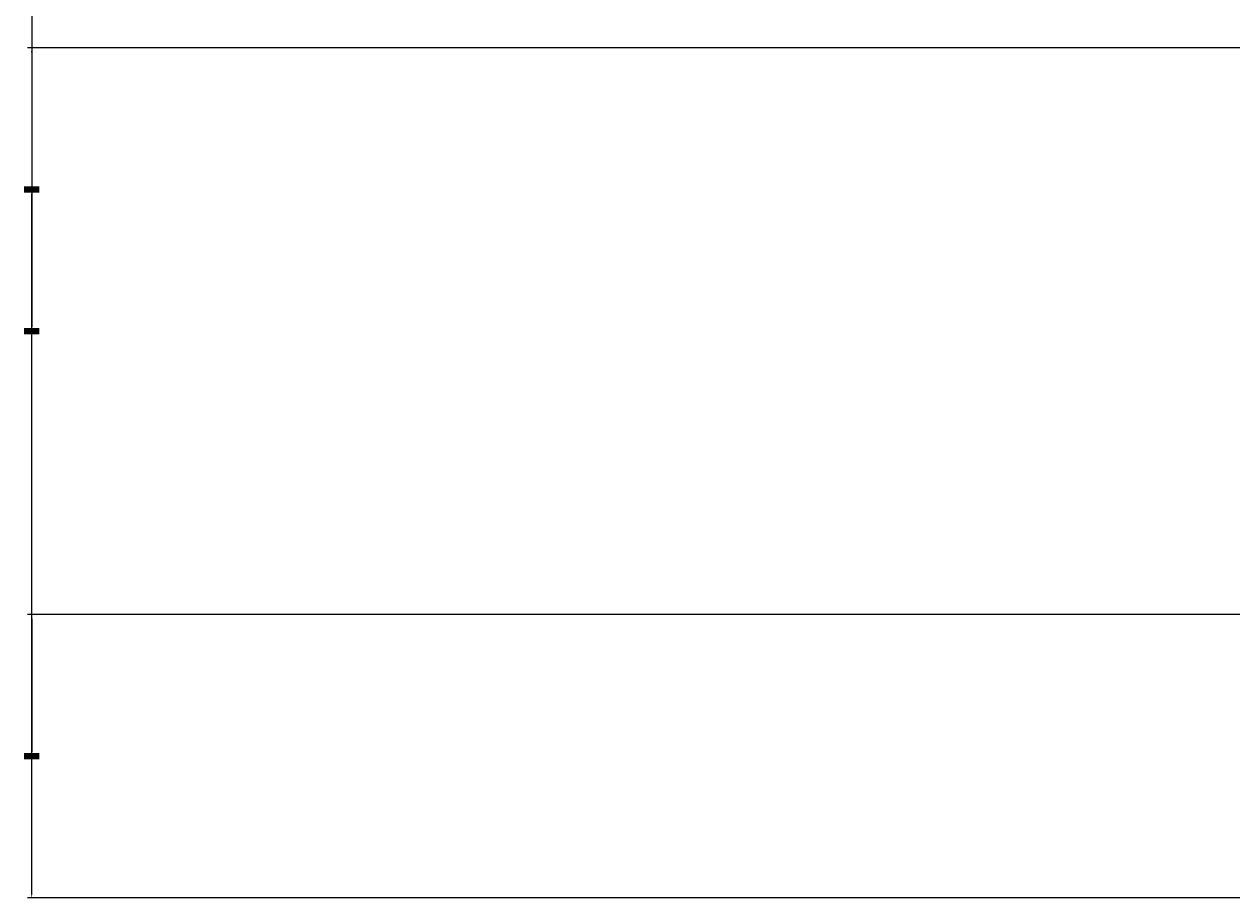
# Model space of a CAD drawing. Units: inches. Extents: x -128 to 854, y -395 to 398.
# Tile 1 of 61: x -128 to -77, y -358 to -321. Entities that reach past the tile are written whole.
import ezdxf

# ---------------------------------------------------------------- set-up
doc = ezdxf.new("R2010")
doc.units = ezdxf.units.IN
doc.header["$MEASUREMENT"] = 0
doc.layers.add('A-ANNO-DIMS', color=2, linetype='Continuous', lineweight=18)
doc.styles.get("Standard").update_dxf_attribs({"font": 'arial.ttf'})
doc.dimstyles.get("Standard").update_dxf_attribs({"dimtxt": 0.18, "dimasz": 0.18, "dimexe": 0.18, "dimexo": 0.0625, "dimgap": 0.09, "dimtad": 0, "dimtih": 1, "dimtoh": 1, "dimdec": 1, "dimzin": 0, "dimdsep": 46, "dimlunit": 4, "dimtxsty": 'Standard', "dimcen": 0.09, "dimclrd": 1, "dimclre": 2, "dimclrt": 6, "dimadec": 0, "dimazin": 0, "dimtfac": 1, "dimtdec": 1, "dimtofl": 0, "dimtmove": 0, "dimatfit": 3, "dimfxl": 1, "dimtfill": 2, "dimtfillclr": 3, "dimtolj": 1, "dimtzin": 0, "dimarcsym": 0})

# ---------------------------------------------------------------- blocks, each defined once
blk = doc.blocks.new('*D121')
at = {"layer": 'A-ANNO-DIMS', "color": 2, "lineweight": -2, "transparency": 16777216}
for p, q in [((-56.223, -298.019), (-128.041, -298.019)), ((-76.223, -358.019), (-128.041, -358.019))]:
    blk.add_line(p, q, dxfattribs=at)
at = {"layer": 'A-ANNO-DIMS', "color": 1, "lineweight": -2, "transparency": 16777216}
for p, q in [((-127.861, -298.199), (-127.861, -327.837)), ((-127.861, -357.839), (-127.861, -328.201))]:
    blk.add_line(p, q, dxfattribs=at)
at = {"layer": 'A-ANNO-DIMS', "color": 1, "transparency": 16777216}
for points in [[(-127.891, -298.199), (-127.831, -298.199), (-127.861, -298.019)], [(-127.891, -357.839), (-127.831, -357.839), (-127.861, -358.019)]]:
    blk.add_solid(points, dxfattribs=at)
at = {"layer": 'Defpoints', "color": 0, "transparency": 16777216}
for p in [(-56.161, -298.019), (-127.861, -358.019), (-76.161, -358.019)]:
    blk.add_point(p, dxfattribs=at)
at = {"layer": 'A-ANNO-DIMS', "color": 6, "transparency": 16777216, "insert": (-127.861, -328.019), "char_height": 0.18, "attachment_point": 5, "bg_fill": 1, "box_fill_scale": 1.25, "bg_fill_color": 3, "bg_fill_transparency": 0}
blk.add_mtext('\\A1;5\'-0"', dxfattribs=at)
blk = doc.blocks.new('*D128')
at = {"layer": 'A-ANNO-DIMS', "color": 2, "lineweight": -2, "transparency": 16777216}
for p, q in [((-17.223, -346.019), (-128.041, -346.019)), ((-17.223, -358.019), (-128.041, -358.019))]:
    blk.add_line(p, q, dxfattribs=at)
at = {"layer": 'A-ANNO-DIMS', "color": 1, "lineweight": -2, "transparency": 16777216}
for p, q in [((-127.861, -346.199), (-127.861, -351.837)), ((-127.861, -357.839), (-127.861, -352.201))]:
    blk.add_line(p, q, dxfattribs=at)
at = {"layer": 'A-ANNO-DIMS', "color": 1, "transparency": 16777216}
for points in [[(-127.891, -346.199), (-127.831, -346.199), (-127.861, -346.019)], [(-127.891, -357.839), (-127.831, -357.839), (-127.861, -358.019)]]:
    blk.add_solid(points, dxfattribs=at)
at = {"layer": 'Defpoints', "color": 0, "transparency": 16777216}
for p in [(-127.861, -346.019), (-17.161, -346.019), (-17.161, -358.019)]:
    blk.add_point(p, dxfattribs=at)
at = {"layer": 'A-ANNO-DIMS', "color": 6, "transparency": 16777216, "insert": (-127.861, -352.019), "char_height": 0.18, "attachment_point": 5, "bg_fill": 1, "box_fill_scale": 1.25, "bg_fill_color": 3, "bg_fill_transparency": 0}
blk.add_mtext('\\A1;1\'-0"', dxfattribs=at)
blk = doc.blocks.new('*D129')
at = {"layer": 'A-ANNO-DIMS', "color": 2, "lineweight": -2, "transparency": 16777216}
for p, q in [((-27.223, -322.019), (-128.041, -322.019)), ((-27.223, -346.019), (-128.041, -346.019))]:
    blk.add_line(p, q, dxfattribs=at)
at = {"layer": 'A-ANNO-DIMS', "color": 1, "lineweight": -2, "transparency": 16777216}
for p, q in [((-127.861, -322.199), (-127.861, -333.837)), ((-127.861, -345.839), (-127.861, -334.201))]:
    blk.add_line(p, q, dxfattribs=at)
at = {"layer": 'A-ANNO-DIMS', "color": 1, "transparency": 16777216}
for points in [[(-127.891, -322.199), (-127.831, -322.199), (-127.861, -322.019)], [(-127.891, -345.839), (-127.831, -345.839), (-127.861, -346.019)]]:
    blk.add_solid(points, dxfattribs=at)
at = {"layer": 'Defpoints', "color": 0, "transparency": 16777216}
for p in [(-127.861, -322.019), (-27.161, -322.019), (-27.161, -346.019)]:
    blk.add_point(p, dxfattribs=at)
at = {"layer": 'A-ANNO-DIMS', "color": 6, "transparency": 16777216, "insert": (-127.861, -334.019), "char_height": 0.18, "attachment_point": 5, "bg_fill": 1, "box_fill_scale": 1.25, "bg_fill_color": 3, "bg_fill_transparency": 0}
blk.add_mtext('\\A1;2\'-0"', dxfattribs=at)

msp = doc.modelspace()

# ---------------------------------------------------------------- dimensions: what is measured, and where the dimension line sits
at = {"layer": 'A-ANNO-DIMS'}
for base, p1, p2, picture, middle in [((-127.861, -358.019), (-56.161, -298.019), (-76.161, -358.019), '*D121', (-127.861, -328.019)), ((-127.861, -322.019), (-27.161, -346.019), (-27.161, -322.019), '*D129', (-127.861, -334.019)), ((-127.861, -346.019), (-17.161, -358.019), (-17.161, -346.019), '*D128', (-127.861, -352.019))]:
    dim = msp.add_linear_dim(base=base, p1=p1, p2=p2, angle=90, dimstyle='Standard', override={"dimdec": 1, "dimlfac": 1, "dimrnd": 0, "dimzin": 1, "dimdsep": 46, "dimlunit": 4, "dimfrac": 2}, dxfattribs=at)
    dim.commit()
    dim.dimension.update_dxf_attribs({"geometry": picture, "text_midpoint": middle})

doc.saveas('drawing.dxf')
